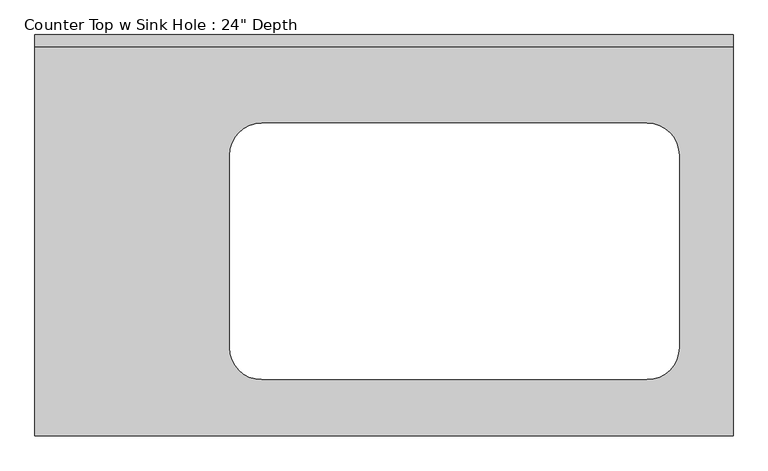
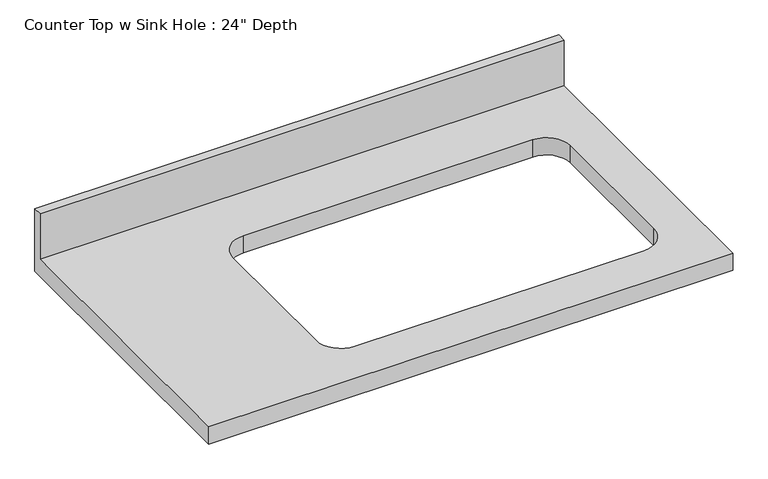
"""IFC4 building model written with IfcOpenShell, lengths in millimetres: furniture geometry."""

from ifc_helpers import new_model, si_unit, frame, origin, place, context, project, spatial, polyline, circle_curve, source, transform, mapped, element, save
from ifc_brep_helpers import plane_surface, revolved_surface, advanced_brep


def furniture_8ade2860(model_context):
    return source(origin(), model_context, "Body", "AdvancedBrep", [
        advanced_brep(
        [(-1200.4622951, -635.0, 914.4), (-95.5622951, -635.0, 914.4), (-95.5622951, -19.05, 914.4), (-1200.4622951, -19.05, 914.4), (-841.4522845, -139.7, 914.4), (-231.8522845, -139.7, 914.4), (-181.0522845, -190.5, 914.4), (-181.0522845, -495.3, 914.4), (-231.8522845, -546.1, 914.4), (-841.4522845, -546.1, 914.4), (-892.2522845, -495.3, 914.4), (-892.2522845, -190.5, 914.4), (-95.5622951, 0.0, 876.3), (-95.5622951, -635.0, 876.3), (-1200.4622951, -635.0, 876.3), (-1200.4622951, 0.0, 876.3), (-231.8522845, -139.7, 876.3), (-841.4522845, -139.7, 876.3), (-892.2522845, -190.5, 876.3), (-892.2522845, -495.3, 876.3), (-841.4522845, -546.1, 876.3), (-231.8522845, -546.1, 876.3), (-181.0522845, -495.3, 876.3), (-181.0522845, -190.5, 876.3), (-1200.4622951, 0.0, 1016.0), (-95.5622951, 0.0, 1016.0), (-1200.4622951, -19.05, 1016.0), (-95.5622951, -19.05, 1016.0)],
        [
            (0, 1),
            (1, 2),
            (2, 3),
            (3, 0),
            (4, 5),
            (5, 6, circle_curve(frame((-231.8522845, -190.5, 914.4), z_axis=(0.0, 0.0, -1.0), x_axis=(1.0, 0.0, 0.0)), 50.8)),
            (6, 7),
            (7, 8, circle_curve(frame((-231.8522845, -495.3, 914.4), z_axis=(0.0, 0.0, -1.0), x_axis=(1.0, 0.0, 0.0)), 50.8)),
            (8, 9),
            (9, 10, circle_curve(frame((-841.4522845, -495.3, 914.4), z_axis=(0.0, 0.0, -1.0), x_axis=(1.0, 0.0, 0.0)), 50.8)),
            (10, 11),
            (11, 4, circle_curve(frame((-841.4522845, -190.5, 914.4), z_axis=(0.0, 0.0, -1.0), x_axis=(1.0, 0.0, 0.0)), 50.8)),
            (12, 13),
            (13, 14),
            (14, 15),
            (15, 12),
            (16, 17),
            (17, 18, circle_curve(frame((-841.4522845, -190.5, 876.3), z_axis=(0.0, 0.0, 1.0), x_axis=(1.0, 0.0, 0.0)), 50.8)),
            (18, 19),
            (19, 20, circle_curve(frame((-841.4522845, -495.3, 876.3), z_axis=(0.0, 0.0, 1.0), x_axis=(1.0, 0.0, 0.0)), 50.8)),
            (20, 21),
            (21, 22, circle_curve(frame((-231.8522845, -495.3, 876.3), z_axis=(0.0, 0.0, 1.0), x_axis=(1.0, 0.0, 0.0)), 50.8)),
            (22, 23),
            (23, 16, circle_curve(frame((-231.8522845, -190.5, 876.3), z_axis=(0.0, 0.0, 1.0), x_axis=(1.0, 0.0, 0.0)), 50.8)),
            (15, 24),
            (24, 25),
            (25, 12),
            (14, 0),
            (3, 26),
            (26, 24),
            (13, 1),
            (25, 27),
            (27, 2),
            (26, 27),
            (4, 17),
            (16, 5),
            (11, 18),
            (10, 19),
            (9, 20),
            (8, 21),
            (7, 22),
            (6, 23),
        ],
        [
            plane_surface(frame((-1200.4622951, 0.0, 914.4), z_axis=(0.0, 0.0, 1.0), x_axis=(-1.0, 0.0, 0.0))),
            plane_surface(frame((-1200.4622951, 0.0, 876.3), z_axis=(0.0, 0.0, -1.0), x_axis=(1.0, 0.0, 0.0))),
            plane_surface(frame((-95.5622951, 0.0, 914.4), z_axis=(0.0, 1.0, 0.0), x_axis=(0.0, 0.0, -1.0))),
            plane_surface(frame((-1200.4622951, 0.0, 914.4), z_axis=(-1.0, 0.0, 0.0), x_axis=(0.0, 0.0, -1.0))),
            plane_surface(frame((-1200.4622951, -635.0, 914.4), z_axis=(0.0, -1.0, 0.0), x_axis=(0.0, 0.0, -1.0))),
            plane_surface(frame((-95.5622951, -635.0, 914.4), z_axis=(1.0, 0.0, 0.0), x_axis=(0.0, 0.0, -1.0))),
            plane_surface(frame((-1200.4622951, 0.0, 1016.0), z_axis=(0.0, 0.0, 1.0), x_axis=(0.0, -1.0, 0.0))),
            plane_surface(frame((-1200.4622951, -19.05, 1016.0), z_axis=(0.0, -1.0, 0.0), x_axis=(0.0, 0.0, -1.0))),
            plane_surface(frame((-231.8522845, -139.7, 914.4), z_axis=(0.0, -1.0, 0.0), x_axis=(0.0, 0.0, -1.0))),
            revolved_surface(polyline([(-790.6522845000001, -190.5, 914.4), (-790.6522845000001, -190.5, 876.3)]), (-841.4522845, -190.5, 876.3), (0.0, 0.0, 1.0)),
            plane_surface(frame((-892.2522845, -190.5, 914.4), z_axis=(1.0, 0.0, 0.0), x_axis=(0.0, 0.0, -1.0))),
            revolved_surface(polyline([(-790.6522845000001, -495.3, 914.4), (-790.6522845000001, -495.3, 876.3)]), (-841.4522845, -495.3, 876.3), (0.0, 0.0, 1.0)),
            plane_surface(frame((-841.4522845, -546.1, 914.4), z_axis=(0.0, 1.0, 0.0), x_axis=(0.0, 0.0, -1.0))),
            revolved_surface(polyline([(-181.05228449999998, -495.3, 914.4), (-181.05228449999998, -495.3, 876.3)]), (-231.8522845, -495.3, 876.3), (0.0, 0.0, 1.0)),
            plane_surface(frame((-181.0522845, -495.3, 914.4), z_axis=(-1.0, 0.0, 0.0), x_axis=(0.0, 0.0, -1.0))),
            revolved_surface(polyline([(-181.05228449999998, -190.5, 914.4), (-181.05228449999998, -190.5, 876.3)]), (-231.8522845, -190.5, 876.3), (0.0, 0.0, 1.0)),
        ],
        [
            (0, [[1, 2, 3, 4], [5, 6, 7, 8, 9, 10, 11, 12]]),
            (1, [[13, 14, 15, 16], [17, 18, 19, 20, 21, 22, 23, 24]]),
            (2, [[-16, 25, 26, 27]]),
            (3, [[-15, 28, -4, 29, 30, -25]]),
            (4, [[-1, -28, -14, 31]]),
            (5, [[-13, -27, 32, 33, -2, -31]]),
            (6, [[-30, 34, -32, -26]]),
            (7, [[-34, -29, -3, -33]]),
            (8, [[35, -17, 36, -5]]),
            (9, [[-35, -12, 37, -18]]),
            (10, [[-37, -11, 38, -19]]),
            (11, [[-38, -10, 39, -20]]),
            (12, [[-39, -9, 40, -21]]),
            (13, [[-40, -8, 41, -22]]),
            (14, [[-41, -7, 42, -23]]),
            (15, [[-36, -24, -42, -6]]),
        ],
    ),
    ])


if __name__ == "__main__":
    model = new_model("IFC4")
    model_context = context("Model", 3, world=origin())
    ifc_project = project(units=[si_unit("LENGTHUNIT", "METRE", prefix="MILLI")], contexts=[model_context])
    site = spatial("IfcSite", under=ifc_project)
    building = spatial("IfcBuilding", under=site)
    placement = place(None, origin())
    furniture_shape = furniture_8ade2860(model_context)
    element("IfcFurniture", 1, ObjectType="Counter Top w Sink Hole : 24\" Depth", at=placement, inside=building, context=model_context, shape_type="MappedRepresentation", body=[
        mapped(furniture_shape, transform((0.0, 0.0, 0.0), x_axis=(1.0, 0.0, 0.0), y_axis=(0.0, 1.0, 0.0), z_axis=(0.0, 0.0, 1.0))),
    ])
    save(model, "model.ifc")

# Revit data of these elements
# Type "Counter Top w Sink Hole : 24\" Depth"
#   Assembly Code = "C1030400"
#   Counter Thickness = 0' - 1 1/2"
#   Depth = 2' - 1"
#   Height = 3' - 0"
#   Length [instance default] = 8' - 0"
#   Sink Location [instance default] = 2' - 0"
#   Sink Location To Wall [instance default] = 0' - 6"
#   Sink Opening Depth [instance default] = 1' - 3"
#   Sink Opening Width [instance default] = 2' - 3"
#   Counter Top Material = none
#   Default Elevation = 0
# Element 1 (IfcFurniture, "Counter Top w Sink Hole : 24\" Depth")
#   Length = 3' - 7 1/2"
#   Sink Location = 2' - 2.13425"
#   Materials on its faces: "Counter Top"
# Materials
#   "Counter Top": class "Wood", colour RGB 226 177 128, transparency 0
